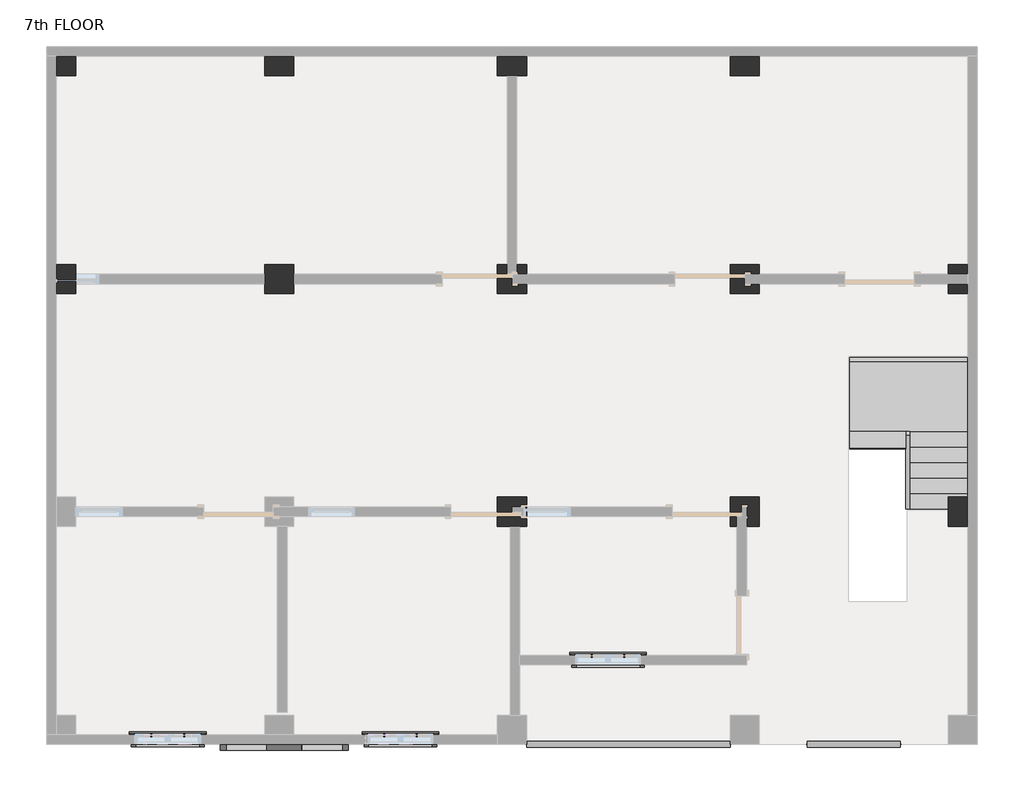
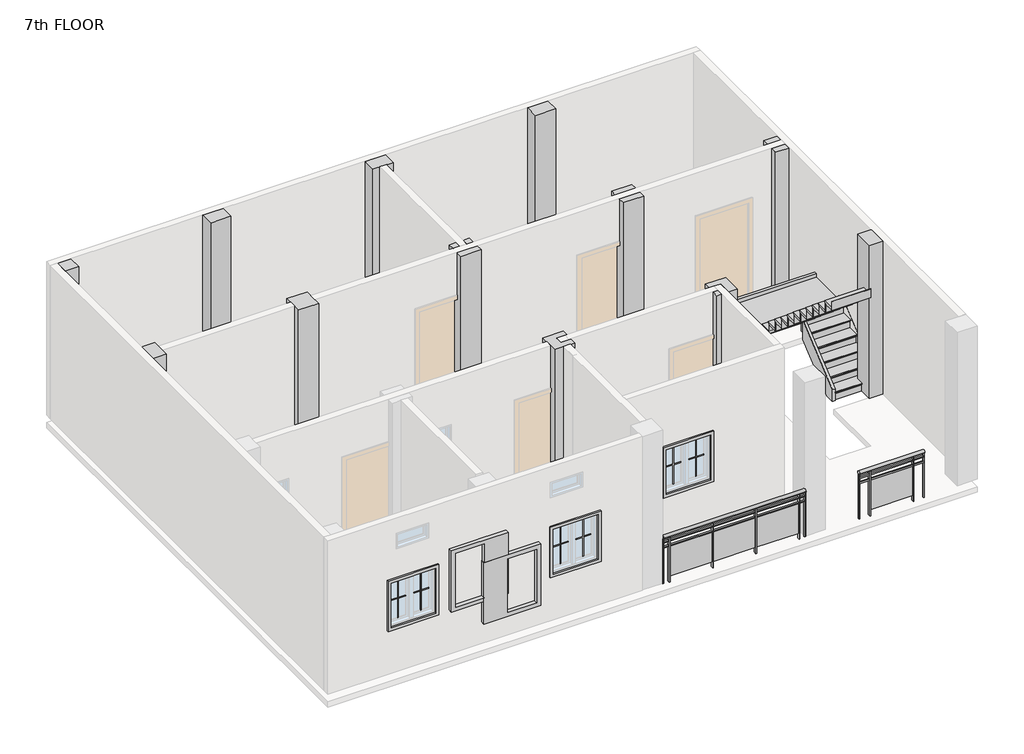
# One storey, part 2 of 2: 12 columns, 12 proxies, 4 members, 2 railings, 1 damper, 1 stair flight.
"""IFC4 building model written with IfcOpenShell, lengths in millimetres."""

from ifc_helpers import new_model, si_unit, point, frame, origin, place, context, project, spatial, polyline, ellipse_curve, trimmed, outline, extrude, faceted_brep, transform, mapped, element, save
from ifc_brep_helpers import plane_surface, extruded_surface, advanced_brep
from components import muntin_pattern_2x2_muntin_pattern_2x2_b3fe6957, muntin_pattern_2x2_muntin_pattern_2x2_3e0ecaf2, trim_window_exterior_flat_with_sill_41619996, trim_window_interior_flat_picture_frame_51c85655, duct_accessories_6_duct_accessories_1_9dfa8ad6, stair_flight_f2d67c03

model = new_model("IFC4")

# Units and contexts
model_context = context("Model", 3, world=origin())
ifc_project = project(units=[si_unit("LENGTHUNIT", "METRE", prefix="MILLI")], contexts=[model_context])

# Site, building, storey
site = spatial("IfcSite", under=ifc_project)
building = spatial("IfcBuilding", under=site)
storey = spatial("IfcBuildingStorey", under=building, Name="7th FLOOR", Elevation=21183.6)

# Proxies
placement = place(None, origin())
muntin_pattern_2x2_muntin_pattern_2x2_shape = muntin_pattern_2x2_muntin_pattern_2x2_b3fe6957(model_context)
element("IfcBuildingElementProxy", 1, Name="Muntin Pattern_2x2 : Muntin Pattern_2x2", ObjectType="Muntin Pattern_2x2 : Muntin Pattern_2x2", at=placement, inside=storey, context=model_context, shape_type="MappedRepresentation", body=[
    mapped(muntin_pattern_2x2_muntin_pattern_2x2_shape, transform((-14441.409625, -253.8184478, 22167.85), x_axis=(1.0, 0.0, 0.0), y_axis=(0.0, 1.0, 0.0), z_axis=(0.0, 0.0, 1.0))),
])
element("IfcBuildingElementProxy", 2, Name="Muntin Pattern_2x2 : Muntin Pattern_2x2", ObjectType="Muntin Pattern_2x2 : Muntin Pattern_2x2", at=placement, inside=storey, context=model_context, shape_type="MappedRepresentation", body=[
    mapped(muntin_pattern_2x2_muntin_pattern_2x2_shape, transform((-11393.409625, -253.8184478, 22167.85), x_axis=(1.0, 0.0, 0.0), y_axis=(0.0, 1.0, 0.0), z_axis=(0.0, 0.0, 1.0))),
])
element("IfcBuildingElementProxy", 3, Name="Muntin Pattern_2x2 : Muntin Pattern_2x2", ObjectType="Muntin Pattern_2x2 : Muntin Pattern_2x2", at=placement, inside=storey, context=model_context, shape_type="MappedRepresentation", body=[
    mapped(muntin_pattern_2x2_muntin_pattern_2x2_shape, transform((-8675.609625, 787.5815522, 22167.85), x_axis=(1.0, 0.0, 0.0), y_axis=(0.0, 1.0, 0.0), z_axis=(0.0, 0.0, 1.0))),
])
muntin_pattern_2x2_muntin_pattern_2x2_2_shape = muntin_pattern_2x2_muntin_pattern_2x2_3e0ecaf2(model_context)
element("IfcBuildingElementProxy", 4, Name="Muntin Pattern_2x2 : Muntin Pattern_2x2", ObjectType="Muntin Pattern_2x2 : Muntin Pattern_2x2", at=placement, inside=storey, context=model_context, shape_type="MappedRepresentation", body=[
    mapped(muntin_pattern_2x2_muntin_pattern_2x2_2_shape, transform((-14012.784625, -253.8184478, 22167.85), x_axis=(-1.0, 0.0, 0.0), y_axis=(0.0, -1.0, 0.0), z_axis=(0.0, 0.0, 1.0))),
])
element("IfcBuildingElementProxy", 5, Name="Muntin Pattern_2x2 : Muntin Pattern_2x2", ObjectType="Muntin Pattern_2x2 : Muntin Pattern_2x2", at=placement, inside=storey, context=model_context, shape_type="MappedRepresentation", body=[
    mapped(muntin_pattern_2x2_muntin_pattern_2x2_2_shape, transform((-10964.784625, -253.8184478, 22167.85), x_axis=(-1.0, 0.0, 0.0), y_axis=(0.0, -1.0, 0.0), z_axis=(0.0, 0.0, 1.0))),
])
element("IfcBuildingElementProxy", 6, Name="Muntin Pattern_2x2 : Muntin Pattern_2x2", ObjectType="Muntin Pattern_2x2 : Muntin Pattern_2x2", at=placement, inside=storey, context=model_context, shape_type="MappedRepresentation", body=[
    mapped(muntin_pattern_2x2_muntin_pattern_2x2_2_shape, transform((-8246.984625, 787.5815522, 22167.85), x_axis=(-1.0, 0.0, 0.0), y_axis=(0.0, -1.0, 0.0), z_axis=(0.0, 0.0, 1.0))),
])
trim_window_exterior_flat_with_sill_shape = trim_window_exterior_flat_with_sill_41619996(model_context)
element("IfcBuildingElementProxy", 7, Name="Trim-Window-Exterior-Flat : with Sill", ObjectType="Trim-Window-Exterior-Flat : with Sill", at=placement, inside=storey, context=model_context, shape_type="MappedRepresentation", body=[
    mapped(trim_window_exterior_flat_with_sill_shape, transform((-14227.097125, -244.2934478, 23012.4), x_axis=(-1.0, 0.0, 0.0), y_axis=(0.0, 0.0, 1.0), z_axis=(0.0, 1.0, 0.0))),
])
element("IfcBuildingElementProxy", 8, Name="Trim-Window-Exterior-Flat : with Sill", ObjectType="Trim-Window-Exterior-Flat : with Sill", at=placement, inside=storey, context=model_context, shape_type="MappedRepresentation", body=[
    mapped(trim_window_exterior_flat_with_sill_shape, transform((-11179.097125, -244.2934478, 23012.4), x_axis=(-1.0, 0.0, 0.0), y_axis=(0.0, 0.0, 1.0), z_axis=(0.0, 1.0, 0.0))),
])
element("IfcBuildingElementProxy", 9, Name="Trim-Window-Exterior-Flat : with Sill", ObjectType="Trim-Window-Exterior-Flat : with Sill", at=placement, inside=storey, context=model_context, shape_type="MappedRepresentation", body=[
    mapped(trim_window_exterior_flat_with_sill_shape, transform((-8461.297125, 797.1065522, 23012.4), x_axis=(-1.0, 0.0, 0.0), y_axis=(0.0, 0.0, 1.0), z_axis=(0.0, 1.0, 0.0))),
])
trim_window_interior_flat_picture_frame_shape = trim_window_interior_flat_picture_frame_51c85655(model_context)
element("IfcBuildingElementProxy", 10, Name="Trim-Window-Interior-Flat : Picture Frame", ObjectType="Trim-Window-Interior-Flat : Picture Frame", at=placement, inside=storey, context=model_context, shape_type="MappedRepresentation", body=[
    mapped(trim_window_interior_flat_picture_frame_shape, transform((-14227.097125, -371.2934478, 23012.4), x_axis=(1.0, 0.0, 0.0), y_axis=(0.0, 0.0, 1.0), z_axis=(0.0, -1.0, 0.0))),
])
element("IfcBuildingElementProxy", 11, Name="Trim-Window-Interior-Flat : Picture Frame", ObjectType="Trim-Window-Interior-Flat : Picture Frame", at=placement, inside=storey, context=model_context, shape_type="MappedRepresentation", body=[
    mapped(trim_window_interior_flat_picture_frame_shape, transform((-11179.097125, -371.2934478, 23012.4), x_axis=(1.0, 0.0, 0.0), y_axis=(0.0, 0.0, 1.0), z_axis=(0.0, -1.0, 0.0))),
])
element("IfcBuildingElementProxy", 12, Name="Trim-Window-Interior-Flat : Picture Frame", ObjectType="Trim-Window-Interior-Flat : Picture Frame", at=placement, inside=storey, context=model_context, shape_type="MappedRepresentation", body=[
    mapped(trim_window_interior_flat_picture_frame_shape, transform((-8461.297125, 670.1065522, 23012.4), x_axis=(1.0, 0.0, 0.0), y_axis=(0.0, 0.0, 1.0), z_axis=(0.0, -1.0, 0.0))),
])

# Columns
element("IfcColumn", 13, ObjectType="column family : column family", at=placement, inside=storey, context=model_context, shape_type="SweptSolid", body=[
    extrude(outline(polyline([(-15433.597125, 8645.7065522), (-15433.597125, 8391.7065522), (-15687.597125, 8391.7065522), (-15687.597125, 8645.7065522), (-15433.597125, 8645.7065522)])), frame((0.0, 0.0, 21188.6), z_axis=(0.0, 0.0, 1.0), x_axis=(1.0, 0.0, 0.0)), (0.0, 0.0, 1.0), 3038.0),
])
element("IfcColumn", 14, ObjectType="column family : column family", at=placement, inside=storey, context=model_context, shape_type="SweptSolid", body=[
    extrude(outline(polyline([(-12576.097125, 5915.2065522), (-12576.097125, 5534.2065522), (-12957.097125, 5534.2065522), (-12957.097125, 5915.2065522), (-12576.097125, 5915.2065522)])), frame((0.0, 0.0, 21188.6), z_axis=(0.0, 0.0, 1.0), x_axis=(1.0, 0.0, 0.0)), (0.0, 0.0, 1.0), 3038.0),
])
element("IfcColumn", 15, ObjectType="column family : column family", at=placement, inside=storey, context=model_context, shape_type="Brep", body=[
    faceted_brep([(-9655.097125, 5915.2065522, 21188.6), (-9528.097125, 5915.2065522, 21188.6), (-9528.097125, 5788.2065522, 21188.6), (-9655.097125, 5788.2065522, 21188.6), (-9528.097125, 5915.2065522, 24226.6), (-9655.097125, 5915.2065522, 24226.6), (-9655.097125, 5788.2065522, 24226.6), (-9528.097125, 5788.2065522, 24226.6)], [[[0, 1, 2, 3]], [[4, 5, 6, 7]], [[0, 3, 6, 5]], [[4, 1, 0, 5]], [[3, 2, 7, 6]], [[1, 4, 7, 2]]]),
    faceted_brep([(-9528.097125, 5534.2065522, 24226.6), (-9528.097125, 5534.2065522, 21188.6), (-9528.097125, 5661.2065522, 21188.6), (-9528.097125, 5661.2065522, 24226.6), (-9909.097125, 5534.2065522, 21188.6), (-9909.097125, 5534.2065522, 24226.6), (-9909.097125, 5915.2065522, 21188.6), (-9909.097125, 5661.2065522, 24226.6), (-9909.097125, 5661.2065522, 23317.2), (-9909.097125, 5788.2065522, 23317.2), (-9909.097125, 5788.2065522, 24226.6), (-9909.097125, 5915.2065522, 24226.6), (-9782.097125, 5915.2065522, 24226.6), (-9782.097125, 5915.2065522, 21188.6), (-9782.097125, 5788.2065522, 21188.6), (-9782.097125, 5788.2065522, 24226.6), (-9782.097125, 5788.2065522, 23317.2), (-9718.597125, 5788.2065522, 21188.6), (-9718.597125, 5788.2065522, 23317.2), (-9718.597125, 5661.2065522, 21188.6), (-9718.597125, 5661.2065522, 23317.2)], [[[0, 1, 2, 3]], [[4, 1, 0, 5]], [[6, 4, 5, 7, 8, 9, 10, 11]], [[6, 11, 12, 13]], [[14, 13, 12, 15, 16]], [[17, 14, 16, 18]], [[19, 20, 8, 7, 3, 2]], [[1, 4, 6, 13, 14, 17, 19, 2]], [[5, 0, 3, 7]], [[12, 11, 10, 15]], [[9, 16, 15, 10]], [[18, 20, 19, 17]], [[20, 18, 16, 9, 8]]]),
])
element("IfcColumn", 16, ObjectType="column family : column family", at=placement, inside=storey, context=model_context, shape_type="Brep", body=[
    faceted_brep([(-6480.097125, 5534.2065522, 21188.6), (-6861.097125, 5534.2065522, 21188.6), (-6861.097125, 5915.2065522, 21188.6), (-6480.097125, 5915.2065522, 21188.6), (-6480.097125, 5788.2065522, 21188.6), (-6670.597125, 5788.2065522, 21188.6), (-6670.597125, 5661.2065522, 21188.6), (-6480.097125, 5661.2065522, 21188.6), (-6480.097125, 5534.2065522, 24226.6), (-6480.097125, 5661.2065522, 24226.6), (-6861.097125, 5534.2065522, 24226.6), (-6861.097125, 5661.2065522, 24226.6), (-6861.097125, 5661.2065522, 23317.2), (-6861.097125, 5788.2065522, 23317.2), (-6861.097125, 5788.2065522, 24226.6), (-6861.097125, 5915.2065522, 24226.6), (-6480.097125, 5915.2065522, 24226.6), (-6670.597125, 5661.2065522, 23317.2), (-6670.597125, 5788.2065522, 23317.2), (-6480.097125, 5788.2065522, 24226.6)], [[[0, 1, 2, 3, 4, 5, 6, 7]], [[8, 0, 7, 9]], [[1, 0, 8, 10]], [[2, 1, 10, 11, 12, 13, 14, 15]], [[3, 2, 15, 16]], [[10, 8, 9, 11]], [[6, 17, 12, 11, 9, 7]], [[13, 18, 5, 4, 19, 14]], [[3, 16, 19, 4]], [[16, 15, 14, 19]], [[18, 17, 6, 5]], [[17, 18, 13, 12]]]),
])
element("IfcColumn", 17, ObjectType="column family : column family", at=placement, inside=storey, context=model_context, shape_type="Brep", body=[
    faceted_brep([(-6480.097125, 2867.2065522, 21188.6), (-6480.097125, 2486.2065522, 21188.6), (-6645.197125, 2486.2065522, 21188.6), (-6645.197125, 2740.2065522, 21188.6), (-6708.697125, 2740.2065522, 21188.6), (-6708.697125, 2613.2065522, 21188.6), (-6772.197125, 2613.2065522, 21188.6), (-6772.197125, 2486.2065522, 21188.6), (-6861.097125, 2486.2065522, 21188.6), (-6861.097125, 2867.2065522, 21188.6), (-6480.097125, 2867.2065522, 24226.6), (-6480.097125, 2486.2065522, 24226.6), (-6861.097125, 2486.2065522, 24226.6), (-6772.197125, 2486.2065522, 24226.6), (-6861.097125, 2613.2065522, 24226.6), (-6861.097125, 2613.2065522, 23317.2), (-6861.097125, 2740.2065522, 23317.2), (-6861.097125, 2740.2065522, 24226.6), (-6861.097125, 2867.2065522, 24226.6), (-6772.197125, 2740.2065522, 24226.6), (-6645.197125, 2740.2065522, 24226.6), (-6645.197125, 2486.2065522, 24226.6), (-6772.197125, 2613.2065522, 24226.6), (-6772.197125, 2613.2065522, 23317.2), (-6772.197125, 2740.2065522, 23317.2), (-6708.697125, 2613.2065522, 23317.2), (-6708.697125, 2740.2065522, 23317.2)], [[[0, 1, 2, 3, 4, 5, 6, 7, 8, 9]], [[1, 0, 10, 11]], [[12, 8, 7, 13]], [[9, 8, 12, 14, 15, 16, 17, 18]], [[0, 9, 18, 10]], [[11, 10, 18, 17, 19, 20, 21]], [[15, 14, 22, 23]], [[17, 16, 24, 19]], [[20, 3, 2, 21]], [[6, 23, 22, 13, 7]], [[14, 12, 13, 22]], [[1, 11, 21, 2]], [[15, 23, 24, 16]], [[25, 23, 6, 5]], [[23, 25, 26, 24]], [[26, 25, 5, 4]], [[24, 26, 4, 3, 20, 19]]]),
])
element("IfcColumn", 18, ObjectType="column family : column family", at=placement, inside=storey, context=model_context, shape_type="Brep", body=[
    faceted_brep([(-9528.097125, 2486.2065522, 21188.6), (-9909.097125, 2486.2065522, 21188.6), (-9909.097125, 2867.2065522, 21188.6), (-9528.097125, 2867.2065522, 21188.6), (-9528.097125, 2740.2065522, 21188.6), (-9566.197125, 2740.2065522, 21188.6), (-9718.597125, 2740.2065522, 21188.6), (-9718.597125, 2613.2065522, 21188.6), (-9566.197125, 2613.2065522, 21188.6), (-9528.097125, 2613.2065522, 21188.6), (-9528.097125, 2486.2065522, 24226.6), (-9528.097125, 2613.2065522, 21488.4), (-9528.097125, 2740.2065522, 21488.4), (-9528.097125, 2867.2065522, 24226.6), (-9528.097125, 2740.2065522, 24226.6), (-9528.097125, 2740.2065522, 23317.2), (-9528.097125, 2613.2065522, 23317.2), (-9528.097125, 2613.2065522, 24226.6), (-9909.097125, 2486.2065522, 24226.6), (-9909.097125, 2867.2065522, 24226.6), (-9566.197125, 2613.2065522, 24226.6), (-9718.597125, 2613.2065522, 24226.6), (-9718.597125, 2740.2065522, 24226.6), (-9566.197125, 2740.2065522, 24226.6), (-9566.197125, 2613.2065522, 23317.2), (-9566.197125, 2613.2065522, 21488.4), (-9566.197125, 2740.2065522, 21488.4), (-9566.197125, 2740.2065522, 23317.2)], [[[0, 1, 2, 3, 4, 5, 6, 7, 8, 9]], [[10, 0, 9, 11, 12, 4, 3, 13, 14, 15, 16, 17]], [[1, 0, 10, 18]], [[2, 1, 18, 19]], [[3, 2, 19, 13]], [[18, 10, 17, 20, 21, 22, 23, 14, 13, 19]], [[11, 9, 8, 7, 21, 20, 17, 16, 24, 25]], [[4, 12, 26, 27, 15, 14, 23, 22, 6, 5]], [[21, 7, 6, 22]], [[25, 24, 27, 26]], [[25, 26, 12, 11]], [[27, 24, 16, 15]]]),
])
element("IfcColumn", 19, ObjectType="column family : column family", at=placement, inside=storey, context=model_context, shape_type="SweptSolid", body=[
    extrude(outline(polyline([(-12576.097125, 8391.7065522), (-12957.097125, 8391.7065522), (-12957.097125, 8645.7065522), (-12576.097125, 8645.7065522), (-12576.097125, 8391.7065522)])), frame((0.0, 0.0, 21188.6), z_axis=(0.0, 0.0, 1.0), x_axis=(1.0, 0.0, 0.0)), (0.0, 0.0, 1.0), 3038.0),
])
element("IfcColumn", 20, ObjectType="column family : column family", at=placement, inside=storey, context=model_context, shape_type="SweptSolid", body=[
    extrude(outline(polyline([(-9528.097125, 8391.7065522), (-9909.097125, 8391.7065522), (-9909.097125, 8645.7065522), (-9528.097125, 8645.7065522), (-9528.097125, 8391.7065522)])), frame((0.0, 0.0, 21188.6), z_axis=(0.0, 0.0, 1.0), x_axis=(1.0, 0.0, 0.0)), (0.0, 0.0, 1.0), 3038.0),
])
element("IfcColumn", 21, ObjectType="column family : column family", at=placement, inside=storey, context=model_context, shape_type="SweptSolid", body=[
    extrude(outline(polyline([(-6480.097125, 8391.7065522), (-6861.097125, 8391.7065522), (-6861.097125, 8645.7065522), (-6480.097125, 8645.7065522), (-6480.097125, 8391.7065522)])), frame((0.0, 0.0, 21188.6), z_axis=(0.0, 0.0, 1.0), x_axis=(1.0, 0.0, 0.0)), (0.0, 0.0, 1.0), 3038.0),
])
element("IfcColumn", 22, ObjectType="column family : column family", at=placement, inside=storey, context=model_context, shape_type="SweptSolid", body=[
    extrude(outline(polyline([(-4003.597125, 5915.2065522), (-3749.597125, 5915.2065522), (-3749.597125, 5788.2065522), (-4003.597125, 5788.2065522), (-4003.597125, 5915.2065522)])), frame((0.0, 0.0, 21188.6), z_axis=(0.0, 0.0, 1.0), x_axis=(1.0, 0.0, 0.0)), (0.0, 0.0, 1.0), 3038.0),
    extrude(outline(polyline([(-3749.597125, 5534.2065522), (-4003.597125, 5534.2065522), (-4003.597125, 5661.2065522), (-3749.597125, 5661.2065522), (-3749.597125, 5534.2065522)])), frame((0.0, 0.0, 21188.6), z_axis=(0.0, 0.0, 1.0), x_axis=(1.0, 0.0, 0.0)), (0.0, 0.0, 1.0), 3038.0),
])
element("IfcColumn", 23, ObjectType="column family : column family", at=placement, inside=storey, context=model_context, shape_type="SweptSolid", body=[
    extrude(outline(polyline([(-4003.597125, 2486.2065522), (-4003.597125, 2867.2065522), (-3749.597125, 2867.2065522), (-3749.597125, 2486.2065522), (-4003.597125, 2486.2065522)])), frame((0.0, 0.0, 21188.6), z_axis=(0.0, 0.0, 1.0), x_axis=(1.0, 0.0, 0.0)), (0.0, 0.0, 1.0), 3038.0),
])
element("IfcColumn", 24, ObjectType="column family : column family", at=placement, inside=storey, context=model_context, shape_type="SweptSolid", body=[
    extrude(outline(polyline([(-15433.597125, 5915.2065522), (-15433.597125, 5534.2065522), (-15687.597125, 5534.2065522), (-15687.597125, 5915.2065522), (-15433.597125, 5915.2065522)])), frame((0.0, 0.0, 21188.6), z_axis=(0.0, 0.0, 1.0), x_axis=(1.0, 0.0, 0.0)), (0.0, 0.0, 1.0), 3038.0),
])

# Damper
duct_accessories_6_duct_accessories_1_shape = duct_accessories_6_duct_accessories_1_9dfa8ad6(model_context)
element("IfcDamper", 25, ObjectType="Duct Accessories 6 : Duct Accessories 1", at=placement, inside=storey, context=model_context, shape_type="MappedRepresentation", body=[
    mapped(duct_accessories_6_duct_accessories_1_shape, transform((0.0, 0.0, 0.0), x_axis=(1.0, 0.0, 0.0), y_axis=(0.0, 1.0, 0.0), z_axis=(0.0, 0.0, 1.0))),
])

# Members
element("IfcMember", 26, ObjectType="Stringer - 2\" Width", at=placement, inside=storey, context=model_context, shape_type="SweptSolid", body=[
    extrude(outline(polyline([(2714.6319226, 21183.6), (2714.6319226, 21420.4438745), (3679.8319226, 22224.7772078), (3679.8319226, 21828.0165243), (2906.5320935, 21183.6), (2714.6319226, 21183.6)])), frame((-4563.0136682, 0.0, 0.0), z_axis=(1.0, 0.0, 0.0), x_axis=(0.0, 1.0, 0.0)), (0.0, 0.0, 1.0), 50.8),
])
element("IfcMember", 27, ObjectType="Stringer - 2\" Width", at=placement, inside=storey, context=model_context, shape_type="SweptSolid", body=[
    extrude(outline(polyline([(-4512.2136682, 3730.6319226), (-4512.2136682, 3679.8319226), (-4563.0136682, 3679.8319226), (-4563.0136682, 3730.6319226), (-4512.2136682, 3730.6319226)])), frame((0.0, 0.0, 21971.0), z_axis=(0.0, 0.0, 1.0), x_axis=(1.0, 0.0, 0.0)), (0.0, 0.0, 1.0), 304.8),
])
element("IfcMember", 28, ObjectType="Stringer - 2\" Width", at=placement, inside=storey, context=model_context, shape_type="SweptSolid", body=[
    extrude(outline(polyline([(2714.6319226, 21183.6), (2714.6319226, 21420.4438745), (3741.0592732, 22275.8), (4217.1720935, 22275.8), (2906.5320935, 21183.6), (2714.6319226, 21183.6)])), frame((-3749.597125, 0.0, 0.0), z_axis=(1.0, 0.0, 0.0), x_axis=(0.0, 1.0, 0.0)), (0.0, 0.0, 1.0), 50.8),
])
element("IfcMember", 29, ObjectType="Stringer - 2\" Width", at=placement, inside=storey, context=model_context, shape_type="SweptSolid", body=[
    extrude(outline(polyline([(-3698.797125, 4695.8319226), (-3698.797125, 4645.0319226), (-5295.0246464, 4645.0319226), (-5295.0246464, 4695.8319226), (-3698.797125, 4695.8319226)])), frame((0.0, 0.0, 21971.0), z_axis=(0.0, 0.0, 1.0), x_axis=(1.0, 0.0, 0.0)), (0.0, 0.0, 1.0), 304.8),
])

# Railings
element("IfcRailing", 30, ObjectType="Glass Panel - Bottom Fill", at=placement, inside=storey, context=model_context, shape_type="SolidModel", body=[
    advanced_brep(
    [(-9528.097125, -333.1934478, 22098.0), (-9528.097125, -409.3934478, 22098.0), (-6861.097125, -333.1934478, 22098.0), (-6861.097125, -409.3934478, 22098.0)],
    [
        (0, 1, ellipse_curve(frame((-9528.097125, -371.2934478, 22098.0), z_axis=(-1.0, 0.0, 0.0), x_axis=(0.0, -1.0, 0.0)), 38.1, 28.575)),
        (1, 0, ellipse_curve(frame((-9528.097125, -371.2934478, 22098.0), z_axis=(-1.0, 0.0, 0.0), x_axis=(0.0, -1.0, 0.0)), 38.1, 28.575)),
        (2, 3, ellipse_curve(frame((-6861.097125, -371.2934478, 22098.0), z_axis=(1.0, 0.0, 0.0), x_axis=(0.0, -1.0, 0.0)), 38.1, 28.575)),
        (3, 2, ellipse_curve(frame((-6861.097125, -371.2934478, 22098.0), z_axis=(1.0, 0.0, 0.0), x_axis=(0.0, -1.0, 0.0)), 38.1, 28.575)),
        (0, 2),
        (3, 1),
    ],
    [
        plane_surface(frame((-9528.097125, -371.2934478, 22098.0), z_axis=(-1.0, 0.0, 0.0), x_axis=(0.0, 1.0, 0.0))),
        plane_surface(frame((-6861.097125, -371.2934478, 22098.0), z_axis=(1.0, 0.0, 0.0), x_axis=(0.0, 1.0, 0.0))),
        extruded_surface(trimmed(ellipse_curve(frame((-6861.097125, -371.2934478, 22098.0), z_axis=(-1.0, 0.0, 0.0), x_axis=(0.0, -1.0, 0.0)), 38.1, 28.575), [point((-6861.097125, -333.1934478, 22098.0))], [point((-6861.097125, -409.3934478, 22098.0))], True, "CARTESIAN"), (-2667.0, 0.0, 0.0), 2667.0),
        extruded_surface(trimmed(ellipse_curve(frame((-6861.097125, -371.2934478, 22098.0), z_axis=(-1.0, 0.0, 0.0), x_axis=(0.0, -1.0, 0.0)), 38.1, 28.575), [point((-6861.097125, -409.3934478, 22098.0))], [point((-6861.097125, -333.1934478, 22098.0))], True, "CARTESIAN"), (-2667.0, 0.0, 0.0), 2667.0),
    ],
    [
        (0, [[1, 2]]),
        (1, [[3, 4]]),
        (2, [[-1, 5, -4, 6]]),
        (3, [[-2, -6, -3, -5]]),
    ],
),
    extrude(outline(polyline([(-9528.097125, -383.9934478), (-9528.097125, -358.5934478), (-6861.097125, -358.5934478), (-6861.097125, -383.9934478), (-9528.097125, -383.9934478)])), frame((0.0, 0.0, 21983.7), z_axis=(0.0, 0.0, 1.0), x_axis=(1.0, 0.0, 0.0)), (0.0, 0.0, 1.0), 25.4),
    extrude(outline(polyline([(-9528.097125, -383.9934478), (-9528.097125, -358.5934478), (-6861.097125, -358.5934478), (-6861.097125, -383.9934478), (-9528.097125, -383.9934478)])), frame((0.0, 0.0, 21882.1), z_axis=(0.0, 0.0, 1.0), x_axis=(1.0, 0.0, 0.0)), (0.0, 0.0, 1.0), 25.4),
    extrude(outline(polyline([(-6981.747125, -396.6934478), (-6981.747125, -345.8934478), (-6969.047125, -345.8934478), (-6969.047125, -396.6934478), (-6981.747125, -396.6934478)])), frame((0.0, 0.0, 21183.6), z_axis=(0.0, 0.0, 1.0), x_axis=(1.0, 0.0, 0.0)), (0.0, 0.0, 1.0), 885.6788223),
    extrude(outline(polyline([(-7788.197125, -364.7582908), (-6975.397125, -364.7582908), (-6975.397125, -371.1082908), (-7788.197125, -371.1082908), (-7788.197125, -364.7582908)])), frame((0.0, 0.0, 21285.2), z_axis=(0.0, 0.0, 1.0), x_axis=(1.0, 0.0, 0.0)), (0.0, 0.0, 1.0), 596.9),
    extrude(outline(polyline([(-7794.547125, -396.6934478), (-7794.547125, -345.8934478), (-7781.847125, -345.8934478), (-7781.847125, -396.6934478), (-7794.547125, -396.6934478)])), frame((0.0, 0.0, 21183.6), z_axis=(0.0, 0.0, 1.0), x_axis=(1.0, 0.0, 0.0)), (0.0, 0.0, 1.0), 885.6788223),
    extrude(outline(polyline([(-8600.997125, -364.7582908), (-7788.197125, -364.7582908), (-7788.197125, -371.1082908), (-8600.997125, -371.1082908), (-8600.997125, -364.7582908)])), frame((0.0, 0.0, 21285.2), z_axis=(0.0, 0.0, 1.0), x_axis=(1.0, 0.0, 0.0)), (0.0, 0.0, 1.0), 596.9),
    extrude(outline(polyline([(-8607.347125, -396.6934478), (-8607.347125, -345.8934478), (-8594.647125, -345.8934478), (-8594.647125, -396.6934478), (-8607.347125, -396.6934478)])), frame((0.0, 0.0, 21183.6), z_axis=(0.0, 0.0, 1.0), x_axis=(1.0, 0.0, 0.0)), (0.0, 0.0, 1.0), 885.6788223),
    extrude(outline(polyline([(-9413.797125, -364.7582908), (-8600.997125, -364.7582908), (-8600.997125, -371.1082908), (-9413.797125, -371.1082908), (-9413.797125, -364.7582908)])), frame((0.0, 0.0, 21285.2), z_axis=(0.0, 0.0, 1.0), x_axis=(1.0, 0.0, 0.0)), (0.0, 0.0, 1.0), 596.9),
    extrude(outline(polyline([(-9420.147125, -396.6934478), (-9420.147125, -345.8934478), (-9407.447125, -345.8934478), (-9407.447125, -396.6934478), (-9420.147125, -396.6934478)])), frame((0.0, 0.0, 21183.6), z_axis=(0.0, 0.0, 1.0), x_axis=(1.0, 0.0, 0.0)), (0.0, 0.0, 1.0), 885.6788223),
    extrude(outline(polyline([(-6873.797125, -380.8184478), (-6873.797125, -361.7684478), (-6854.747125, -361.7684478), (-6854.747125, -380.8184478), (-6873.797125, -380.8184478)])), frame((0.0, 0.0, 21183.6), z_axis=(0.0, 0.0, 1.0), x_axis=(1.0, 0.0, 0.0)), (0.0, 0.0, 1.0), 885.6788223),
    extrude(outline(polyline([(-9534.447125, -380.8184478), (-9534.447125, -361.7684478), (-9515.397125, -361.7684478), (-9515.397125, -380.8184478), (-9534.447125, -380.8184478)])), frame((0.0, 0.0, 21183.6), z_axis=(0.0, 0.0, 1.0), x_axis=(1.0, 0.0, 0.0)), (0.0, 0.0, 1.0), 885.6788223),
])
element("IfcRailing", 31, ObjectType="Glass Panel - Bottom Fill", at=placement, inside=storey, context=model_context, shape_type="SolidModel", body=[
    advanced_brep(
    [(-5851.447125, -333.1934478, 22098.0), (-5851.447125, -409.3934478, 22098.0), (-4632.247125, -333.1934478, 22098.0), (-4632.247125, -409.3934478, 22098.0)],
    [
        (0, 1, ellipse_curve(frame((-5851.447125, -371.2934478, 22098.0), z_axis=(-1.0, 0.0, 0.0), x_axis=(0.0, -1.0, 0.0)), 38.1, 28.575)),
        (1, 0, ellipse_curve(frame((-5851.447125, -371.2934478, 22098.0), z_axis=(-1.0, 0.0, 0.0), x_axis=(0.0, -1.0, 0.0)), 38.1, 28.575)),
        (2, 3, ellipse_curve(frame((-4632.247125, -371.2934478, 22098.0), z_axis=(1.0, 0.0, 0.0), x_axis=(0.0, -1.0, 0.0)), 38.1, 28.575)),
        (3, 2, ellipse_curve(frame((-4632.247125, -371.2934478, 22098.0), z_axis=(1.0, 0.0, 0.0), x_axis=(0.0, -1.0, 0.0)), 38.1, 28.575)),
        (0, 2),
        (3, 1),
    ],
    [
        plane_surface(frame((-5851.447125, -371.2934478, 22098.0), z_axis=(-1.0, 0.0, 0.0), x_axis=(0.0, 1.0, 0.0))),
        plane_surface(frame((-4632.247125, -371.2934478, 22098.0), z_axis=(1.0, 0.0, 0.0), x_axis=(0.0, 1.0, 0.0))),
        extruded_surface(trimmed(ellipse_curve(frame((-4632.247125, -371.2934478, 22098.0), z_axis=(-1.0, 0.0, 0.0), x_axis=(0.0, -1.0, 0.0)), 38.1, 28.575), [point((-4632.247125, -333.1934478, 22098.0))], [point((-4632.247125, -409.3934478, 22098.0))], True, "CARTESIAN"), (-1219.1999999999998, 0.0, 0.0), 1219.1999999999998),
        extruded_surface(trimmed(ellipse_curve(frame((-4632.247125, -371.2934478, 22098.0), z_axis=(-1.0, 0.0, 0.0), x_axis=(0.0, -1.0, 0.0)), 38.1, 28.575), [point((-4632.247125, -409.3934478, 22098.0))], [point((-4632.247125, -333.1934478, 22098.0))], True, "CARTESIAN"), (-1219.1999999999998, 0.0, 0.0), 1219.1999999999998),
    ],
    [
        (0, [[1, 2]]),
        (1, [[3, 4]]),
        (2, [[-1, 5, -4, 6]]),
        (3, [[-2, -6, -3, -5]]),
    ],
),
    extrude(outline(polyline([(-5851.447125, -383.9934478), (-5851.447125, -358.5934478), (-4632.247125, -358.5934478), (-4632.247125, -383.9934478), (-5851.447125, -383.9934478)])), frame((0.0, 0.0, 21983.7), z_axis=(0.0, 0.0, 1.0), x_axis=(1.0, 0.0, 0.0)), (0.0, 0.0, 1.0), 25.4),
    extrude(outline(polyline([(-5851.447125, -383.9934478), (-5851.447125, -358.5934478), (-4632.247125, -358.5934478), (-4632.247125, -383.9934478), (-5851.447125, -383.9934478)])), frame((0.0, 0.0, 21882.1), z_axis=(0.0, 0.0, 1.0), x_axis=(1.0, 0.0, 0.0)), (0.0, 0.0, 1.0), 25.4),
    extrude(outline(polyline([(-4841.797125, -396.6934478), (-4841.797125, -345.8934478), (-4829.097125, -345.8934478), (-4829.097125, -396.6934478), (-4841.797125, -396.6934478)])), frame((0.0, 0.0, 21183.6), z_axis=(0.0, 0.0, 1.0), x_axis=(1.0, 0.0, 0.0)), (0.0, 0.0, 1.0), 885.6788223),
    extrude(outline(polyline([(-5648.247125, -364.7582908), (-4835.447125, -364.7582908), (-4835.447125, -371.1082908), (-5648.247125, -371.1082908), (-5648.247125, -364.7582908)])), frame((0.0, 0.0, 21285.2), z_axis=(0.0, 0.0, 1.0), x_axis=(1.0, 0.0, 0.0)), (0.0, 0.0, 1.0), 596.9),
    extrude(outline(polyline([(-5654.597125, -396.6934478), (-5654.597125, -345.8934478), (-5641.897125, -345.8934478), (-5641.897125, -396.6934478), (-5654.597125, -396.6934478)])), frame((0.0, 0.0, 21183.6), z_axis=(0.0, 0.0, 1.0), x_axis=(1.0, 0.0, 0.0)), (0.0, 0.0, 1.0), 885.6788223),
    extrude(outline(polyline([(-4644.947125, -380.8184478), (-4644.947125, -361.7684478), (-4625.897125, -361.7684478), (-4625.897125, -380.8184478), (-4644.947125, -380.8184478)])), frame((0.0, 0.0, 21183.6), z_axis=(0.0, 0.0, 1.0), x_axis=(1.0, 0.0, 0.0)), (0.0, 0.0, 1.0), 885.6788223),
    extrude(outline(polyline([(-5857.797125, -380.8184478), (-5857.797125, -361.7684478), (-5838.747125, -361.7684478), (-5838.747125, -380.8184478), (-5857.797125, -380.8184478)])), frame((0.0, 0.0, 21183.6), z_axis=(0.0, 0.0, 1.0), x_axis=(1.0, 0.0, 0.0)), (0.0, 0.0, 1.0), 885.6788223),
])

# Stair flight
stair_flight_shape = stair_flight_f2d67c03(model_context)
element("IfcStairFlight", 32, ObjectType="2\" Tread 1\" Nosing 1/4\" Riser", at=placement, inside=storey, context=model_context, shape_type="MappedRepresentation", body=[
    mapped(stair_flight_shape, transform((0.0, 0.0, 0.0), x_axis=(1.0, 0.0, 0.0), y_axis=(0.0, 1.0, 0.0), z_axis=(0.0, 0.0, 1.0))),
])

save(model, "model.ifc")

# Revit data of these elements
# Type "Muntin Pattern_2x2 : Muntin Pattern_2x2"
#   Width [instance default] = 4' - 0"
#   Thickness = 0' - 0 1/2"
#   Height [instance default] = 4' - 0"
#   Distance = 0' - 0 3/4"
#   Interior Material [instance default] = none
#   Exterior Material [instance default] = none
#   Default Elevation = 0
# Type "Trim-Window-Exterior-Flat : with Sill"
#   Trim Width = 0' - 2 1/4"
#   Trim Thickness_Picture Frame = 0' - 1 1/4"
#   Trim Thickness_with Sill = 0' - 0 3/4"
#   Sill Thickness = 0' - 1 1/4"
#   Opening Width [instance default] = 2' - 0"
#   Opening Height [instance default] = 3' - 0"
#   Default Elevation = 4' - 0"
#   Sill = yes
#   Picture Frame = no
#   Trim Material [instance default] = none
# Type "Trim-Window-Interior-Flat : Picture Frame"
#   Trim Thickness_Picture Frame = 0' - 1 1/4"
#   Trim Width = 0' - 2 1/4"
#   Trim Thickness_with Sill = 0' - 0 3/4"
#   Sill Thickness = 0' - 1 1/4"
#   Opening Width [instance default] = 2' - 0"
#   Opening Height [instance default] = 3' - 0"
#   Default Elevation = 4' - 0"
#   Sill = no
#   Picture Frame = yes
#   Trim Material [instance default] = none
# Type "column family : column family"
#   w2 [instance default] = 0' - 9.88189"
#   w1 [instance default] = 0' - 9.01575"
#   Depth = 1' - 11.62205"
#   Width = 1' - 11.62205"
# Type "Glass Panel - Bottom Fill"
#   Assembly Code = "C2010400"
#   built-in parameter 1008612 = 0.0416667 (stored number, unit not read)
#   built-in parameter 1008611 = 0.0416667 (stored number, unit not read)
#   built-in parameter 1008609 = 0.333333 (stored number, unit not read)
#   built-in parameter 1008604 = 0.166667 (stored number, unit not read)
#   built-in parameter 1008603 = 0.166667 (stored number, unit not read)
#   Railing Height = 3' - 0"
#   built-in parameter 1008630 = 2
#   built-in parameter 1008610 = 2
#   built-in parameter 1008618 = Baluster - Square : 3/4"
# Elements 1, 2, 3, 4, 5, 6 (IfcBuildingElementProxy, "Muntin Pattern_2x2 : Muntin Pattern_2x2")
#   Width = 0' - 11 5/8"
#   Height = 2' - 6 1/2"
#   Interior Material = Wood - Stained
#   Exterior Material = Clad - White
#   Phase Created = New Construction
#   Materials on its faces: "Clad - White", "Wood - Stained"
# Elements 7, 8, 9 (IfcBuildingElementProxy, "Trim-Window-Exterior-Flat : with Sill")
#   Opening Width = 2' - 10"
#   Opening Height = 3' - 0"
#   Trim Material = Clad - White
#   Phase Created = New Construction
#   Materials on its faces: "Clad - White"
# Elements 10, 11, 12 (IfcBuildingElementProxy, "Trim-Window-Interior-Flat : Picture Frame")
#   Opening Width = 2' - 10"
#   Opening Height = 3' - 0"
#   Trim Material = Wood - Stained
#   Phase Created = New Construction
#   Materials on its faces: "Wood - Stained"
# Elements 13, 14, 15, 19, 20, 21 (IfcColumn, "column family : column family")
#   w2 = 1' - 3"
#   w1 = 1' - 3"
#   Phase Created = New Construction
#   Materials on its faces: "Default Wall"
# Elements 16, 22, 23 (IfcColumn, "column family : column family")
#   w2 = 1' - 3"
#   w1 = 1' - 3"
#   Phase Created = New Construction
#   Materials on its faces: "grey", "Default Wall"
# Elements 17, 18 (IfcColumn, "column family : column family")
#   w2 = 1' - 3"
#   w1 = 1' - 3"
#   Phase Created = New Construction
#   Materials on its faces: "Default Wall", "inside wall"
# Element 24 (IfcColumn, "column family : column family")
#   w2 = 1' - 3"
#   w1 = 1' - 3"
#   Phase Created = New Construction
#   Materials on its faces: "inside wall", "Default Wall"
# Element 25 (IfcDamper, "Duct Accessories 6 : Duct Accessories 1")
#   Mark = "6"
#   Phase Created = New Construction
#   Materials on its faces: "border"
# Elements 26, 27, 28, 29 (IfcMember, "Stringer - 2\" Width")
#   Phase Created = New Construction
# Elements 30, 31 (IfcRailing, "Glass Panel - Bottom Fill")
#   Phase Created = New Construction
#   Materials on its faces: "Glass"
# Element 32 (IfcStairFlight, "2\" Tread 1\" Nosing 1/4\" Riser")
#   Phase Created = New Construction
# Materials
#   "Clad - White": class "Wood", colour RGB 242 242 238, transparency 0, Cost = 0
#   "Wood - Stained": class "Wood", colour RGB 224 178 126, transparency 0, Cost = 0
#   "Default Wall": colour RGB 128 128 128, transparency 0, Cost = 0
#   "grey": class "Generic", colour RGB 80 80 80, transparency 0, Cost = 0
#   "inside wall": class "Generic", colour RGB 199 224 95, transparency 0, Cost = 0
#   "border": class "Generic", colour RGB 144 144 144, transparency 0, Cost = 0
#   "Glass": class "Glass", colour RGB 0 128 192, transparency 0.75, Description = "Soda Lime Glass", Cost = 0
